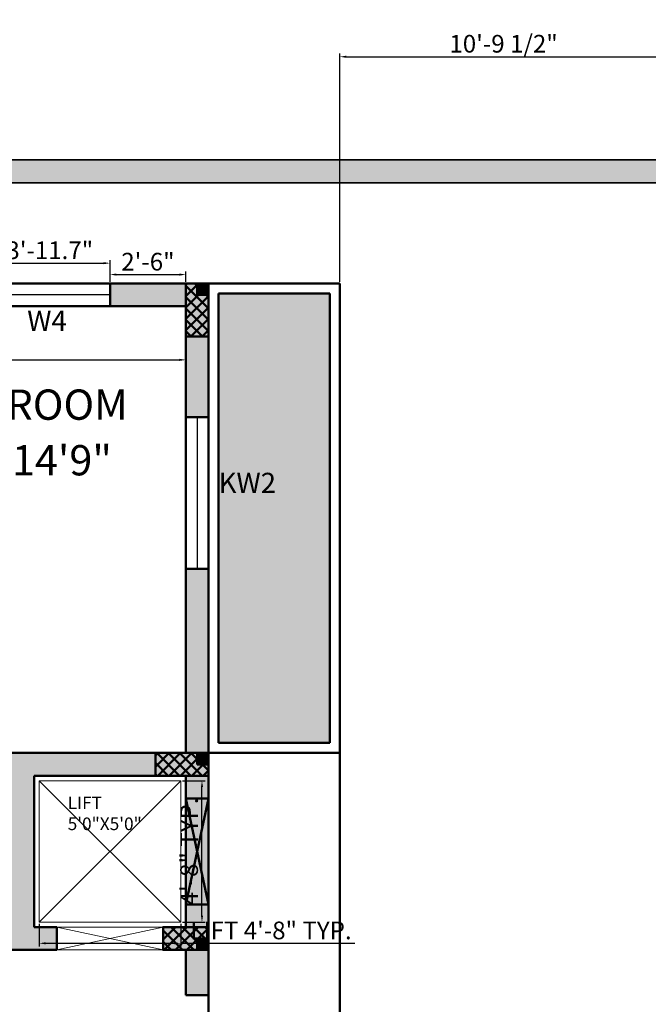
# Model space of a CAD drawing. Units: inches. Extents: x 1749 to 3550, y 1117 to 2383.
# Tile 8 of 15: x 2038 to 2287, y 1993 to 2383. Entities that reach past the tile are written whole.
import ezdxf

# ---------------------------------------------------------------- set-up
doc = ezdxf.new("R2010")
doc.units = ezdxf.units.IN
for name, color, linetype, lineweight in [('A-ANNO-DIMS', 2, 'Continuous', 18), ('A-ANNO-TEXT', 3, 'Continuous', 18), ('A-AREA-IDEN', 7, 'Continuous', 18), ('A-COLS', 10, 'Continuous', 50), ('A-EQPM', 8, 'Continuous', 18), ('A-GLAZ', 4, 'Continuous', 25), ('A-WALL', 7, 'Continuous', 50), ('A-WALL-PATT', 8, 'Continuous', 13), ('C-PROP', 8, 'Continuous', 35)]:
    doc.layers.add(name, color=color, linetype=linetype, lineweight=lineweight)
doc.styles.get("Standard").update_dxf_attribs({"font": 'arial.ttf'})
doc.dimstyles.new('ISO-25', dxfattribs={"dimtxt": 7, "dimasz": 2.5, "dimexe": 1.25, "dimexo": 0.625, "dimtad": 1, "dimdec": 1, "dimlunit": 3, "dimtxsty": 'Standard', "dimcen": 2.5, "dimadec": 0, "dimazin": 0, "dimtfac": 1, "dimtdec": 1, "dimtmove": 0, "dimatfit": 3, "dimfxl": 1, "dimarcsym": 0})

# ---------------------------------------------------------------- blocks, each defined once
blk = doc.blocks.new('*D5')
at = {"layer": 'A-ANNO-DIMS', "color": 0, "lineweight": -2, "transparency": 16777216}
for p, q in [((1868.6, 2249.04), (1868.6, 2249.66)), ((1871.1, 2248.41), (2101.6, 2248.41)), ((2104.1, 2249.04), (2104.1, 2249.66))]:
    blk.add_line(p, q, dxfattribs=at)
at = {"layer": 'A-ANNO-DIMS', "color": 0, "transparency": 16777216}
for points in [[(1871.1, 2248.83), (1871.1, 2247.99), (1868.6, 2248.41)], [(2101.6, 2248.83), (2101.6, 2247.99), (2104.1, 2248.41)]]:
    blk.add_solid(points, dxfattribs=at)
at = {"layer": 'Defpoints', "color": 0, "transparency": 16777216}
for p in [(1868.6, 2248.41), (2104.1, 2248.41), (2104.1, 2248.41)]:
    blk.add_point(p, dxfattribs=at)
at = {"layer": 'A-ANNO-DIMS', "color": 0, "transparency": 16777216, "insert": (1986.35, 2252.61), "char_height": 7, "attachment_point": 5}
blk.add_mtext('19\'-7.5"', dxfattribs=at)
blk = doc.blocks.new('*D76')
at = {"layer": 'A-ANNO-DIMS', "color": 0, "lineweight": -2, "ltscale": 0.5, "transparency": 16777216}
for p, q in [((2026.42, 2279.29), (2026.42, 2287.96)), ((2028.92, 2286.71), (2071.6, 2286.71)), ((2074.1, 2279.29), (2074.1, 2287.96))]:
    blk.add_line(p, q, dxfattribs=at)
at = {"layer": 'A-ANNO-DIMS', "color": 0, "ltscale": 0.5, "transparency": 16777216}
for points in [[(2028.92, 2287.12), (2028.92, 2286.29), (2026.42, 2286.71)], [(2071.6, 2287.12), (2071.6, 2286.29), (2074.1, 2286.71)]]:
    blk.add_solid(points, dxfattribs=at)
at = {"layer": 'Defpoints', "color": 0, "ltscale": 0.5, "transparency": 16777216}
for p in [(2074.1, 2286.71), (2026.42, 2278.66), (2074.1, 2278.66)]:
    blk.add_point(p, dxfattribs=at)
at = {"layer": 'A-ANNO-DIMS', "color": 0, "ltscale": 0.5, "transparency": 16777216, "insert": (2050.26, 2290.91), "char_height": 7, "attachment_point": 5}
blk.add_mtext('3\'-11.7"', dxfattribs=at)
blk = doc.blocks.new('*D77')
at = {"layer": 'A-ANNO-DIMS', "color": 0, "lineweight": -2, "ltscale": 0.5, "transparency": 16777216}
for p, q in [((2074.1, 2279.29), (2074.1, 2283.44)), ((2076.6, 2282.19), (2101.6, 2282.19)), ((2104.1, 2279.29), (2104.1, 2283.44))]:
    blk.add_line(p, q, dxfattribs=at)
at = {"layer": 'A-ANNO-DIMS', "color": 0, "ltscale": 0.5, "transparency": 16777216}
for points in [[(2076.6, 2282.61), (2076.6, 2281.77), (2074.1, 2282.19)], [(2101.6, 2282.61), (2101.6, 2281.77), (2104.1, 2282.19)]]:
    blk.add_solid(points, dxfattribs=at)
at = {"layer": 'Defpoints', "color": 0, "ltscale": 0.5, "transparency": 16777216}
for p in [(2104.1, 2282.19), (2074.1, 2278.66), (2104.1, 2278.66)]:
    blk.add_point(p, dxfattribs=at)
at = {"layer": 'A-ANNO-DIMS', "color": 0, "ltscale": 0.5, "transparency": 16777216, "insert": (2089.1, 2286.39), "char_height": 7, "attachment_point": 5}
blk.add_mtext('2\'-6"', dxfattribs=at)
blk = doc.blocks.new('LIFT-A')
at = {"ltscale": 0.2}
for p, q in [((0, 56), (56, 56)), ((0, 56), (0, 0)), ((56, 56), (0, 0)), ((0, 56), (56, 0)), ((56, 56), (56, 0)), ((0, 0), (56, 0))]:
    blk.add_line(p, q, dxfattribs=at)
blk = doc.blocks.new('*D153')
at = {"layer": 'A-ANNO-DIMS', "color": 0, "lineweight": -2, "ltscale": 0.5, "transparency": 16777216}
for p, q in [((2046.1, 2025.04), (2046.1, 2016.01)), ((2102.1, 2025.04), (2102.1, 2016.01)), ((2048.6, 2017.26), (2099.6, 2017.26)), ((2102.1, 2017.26), (2171.03, 2017.26))]:
    blk.add_line(p, q, dxfattribs=at)
at = {"layer": 'A-ANNO-DIMS', "color": 0, "ltscale": 0.5, "transparency": 16777216}
for points in [[(2048.6, 2017.68), (2048.6, 2016.84), (2046.1, 2017.26)], [(2099.6, 2017.68), (2099.6, 2016.84), (2102.1, 2017.26)]]:
    blk.add_solid(points, dxfattribs=at)
at = {"layer": 'Defpoints', "color": 0, "ltscale": 0.5, "transparency": 16777216}
for p in [(2046.1, 2025.66), (2102.1, 2025.66), (2102.1, 2017.26)]:
    blk.add_point(p, dxfattribs=at)
at = {"layer": 'A-ANNO-DIMS', "color": 0, "ltscale": 0.5, "transparency": 16777216, "insert": (2137.82, 2021.46), "char_height": 7, "attachment_point": 5}
blk.add_mtext('LIFT 4\'-8" TYP.', dxfattribs=at)
blk = doc.blocks.new('*D154')
at = {"layer": 'A-ANNO-DIMS', "color": 0, "lineweight": -2, "ltscale": 0.5, "transparency": 16777216}
for p, q in [((2102.73, 2081.66), (2111.75, 2081.66)), ((2110.5, 2028.16), (2110.5, 2079.16)), ((2102.73, 2025.66), (2111.75, 2025.66))]:
    blk.add_line(p, q, dxfattribs=at)
at = {"layer": 'A-ANNO-DIMS', "color": 0, "ltscale": 0.5, "transparency": 16777216}
for points in [[(2110.09, 2079.16), (2110.92, 2079.16), (2110.5, 2081.66)], [(2110.09, 2028.16), (2110.92, 2028.16), (2110.5, 2025.66)]]:
    blk.add_solid(points, dxfattribs=at)
at = {"layer": 'Defpoints', "color": 0, "ltscale": 0.5, "transparency": 16777216}
for p in [(2102.1, 2081.66), (2110.5, 2081.66), (2102.1, 2025.66)]:
    blk.add_point(p, dxfattribs=at)
at = {"layer": 'A-ANNO-DIMS', "color": 0, "ltscale": 0.5, "transparency": 16777216, "insert": (2106.31, 2053.66), "char_height": 7, "attachment_point": 5, "rotation": 90}
blk.add_mtext('4\'-8" TYP.', dxfattribs=at)
blk = doc.blocks.new('*D164')
at = {"layer": 'A-ANNO-DIMS', "color": 0, "lineweight": -2, "ltscale": 0.5, "transparency": 16777216}
for p, q in [((2165.1, 2279.29), (2165.1, 2369.73)), ((2167.6, 2368.48), (2292.1, 2368.48)), ((2294.6, 2278.29), (2294.6, 2369.73))]:
    blk.add_line(p, q, dxfattribs=at)
at = {"layer": 'A-ANNO-DIMS', "color": 0, "ltscale": 0.5, "transparency": 16777216}
for points in [[(2167.6, 2368.9), (2167.6, 2368.06), (2165.1, 2368.48)], [(2292.1, 2368.9), (2292.1, 2368.06), (2294.6, 2368.48)]]:
    blk.add_solid(points, dxfattribs=at)
at = {"layer": 'Defpoints', "color": 0, "ltscale": 0.5, "transparency": 16777216}
for p in [(2294.6, 2368.48), (2165.1, 2278.66), (2294.6, 2277.66)]:
    blk.add_point(p, dxfattribs=at)
at = {"layer": 'A-ANNO-DIMS', "color": 0, "ltscale": 0.5, "transparency": 16777216, "insert": (2229.85, 2372.73), "char_height": 7, "attachment_point": 5}
blk.add_mtext('10\'-9 1/2"', dxfattribs=at)

msp = doc.modelspace()

# ---------------------------------------------------------------- hatches: boundary and pattern name
at = {"layer": 'A-COLS'}
h = msp.add_hatch(dxfattribs=at)
h.set_pattern_fill('ANSI37', color=256, angle=-90)
h.set_pattern_definition([(315, (332.5445, 4525.2253), (2.245064, 2.245064), []), (45, (332.5445, 4525.2253), (-2.245064, 2.245064), [])])
h.paths.add_polyline_path([(2113.1, 2278.66), (2104.1, 2278.66), (2104.1, 2257.66), (2113.1, 2257.66)])
h = msp.add_hatch(color=256, dxfattribs=at)
h.dxf.hatch_style = 1
h.paths.add_polyline_path([(2108.6, 2274.16), (2113.1, 2274.16), (2113.1, 2278.66), (2108.6, 2278.66)])
h = msp.add_hatch(dxfattribs=at)
h.set_pattern_fill('ANSI37', color=256)
h.set_pattern_definition([(45, (-154.4595, 312.1017), (-2.245064, 2.245064), []), (135, (-154.4595, 312.1017), (-2.245064, -2.245064), [])])
h.paths.add_polyline_path([(2092.1, 2092.66), (2092.1, 2083.66), (2113.1, 2083.66), (2113.1, 2092.66)])
h = msp.add_hatch(color=256, dxfattribs=at)
h.dxf.hatch_style = 1
h.paths.add_polyline_path([(2108.6, 2088.16), (2113.1, 2088.16), (2113.1, 2092.66), (2108.6, 2092.66)])
h = msp.add_hatch(dxfattribs=at)
h.set_pattern_fill('ANSI37', color=256)
h.paths.add_polyline_path([(2113.1, 2023.66), (2095.1, 2023.66), (2095.1, 2014.66), (2108.6, 2014.66), (2108.6, 2019.16), (2113.1, 2019.16)])
h = msp.add_hatch(color=256, dxfattribs=at)
h.dxf.hatch_style = 1
h.paths.add_polyline_path([(2108.6, 2014.66), (2113.1, 2014.66), (2113.1, 2019.16), (2108.6, 2019.16)])
at = {"layer": 'A-WALL-PATT', "ltscale": 0.5}
h = msp.add_hatch(color=256, dxfattribs=at)
h.dxf.hatch_style = 1
h.paths.add_polyline_path([(2612.84, 2327.58), (1804.37, 2327.58), (1804.37, 1803), (2612.84, 1803), (2612.84, 2093.66), (2603.84, 2093.66), (2603.84, 1812), (1813.37, 1812), (1813.37, 2318.58), (2603.84, 2318.58), (2603.84, 2268.45), (2612.84, 2268.45)])
at = {"layer": 'A-WALL-PATT'}
h = msp.add_hatch(color=256, dxfattribs=at)
h.dxf.hatch_style = 1
h.paths.add_polyline_path([(2113.1, 2278.66), (2074.1, 2278.66), (2074.1, 2269.66), (2104.1, 2269.66), (2104.1, 2225.66), (2113.1, 2225.66)])
h = msp.add_hatch(color=256, dxfattribs=at)
h.dxf.hatch_style = 1
h.paths.add_polyline_path([(2161.1, 2274.66), (2117.1, 2274.66), (2117.1, 2096.66), (2161.1, 2096.66)])
h.paths.add_polyline_path([(2161.1, 1944.66), (2117.1, 1944.66), (2117.1, 1853.66), (2161.1, 1853.66)])
h = msp.add_hatch(color=256, dxfattribs=at)
h.dxf.hatch_style = 1
h.paths.add_polyline_path([(2113.1, 2092.66), (2104.1, 2092.66), (1927.1, 2092.66), (1927.1, 2181.16), (1868.6, 2181.16), (1868.6, 2187.16), (1859.6, 2187.16), (1859.6, 2170.66), (1868.6, 2170.66), (1868.6, 2176.66), (1922.6, 2176.66), (1922.6, 2092.66), (1868.6, 2092.66), (1868.6, 2110.66), (1859.6, 2110.66), (1859.6, 2083.66), (1922.6, 2083.66), (1922.6, 2065.66), (1927.1, 2065.66), (1927.1, 2083.66), (2035.1, 2083.66), (2035.1, 2023.66), (2029.1, 2023.66), (2029.1, 2014.66), (2053.1, 2014.66), (2053.1, 2023.66), (2044.1, 2023.66), (2044.1, 2083.66), (2104.1, 2083.66), (2104.1, 2023.66), (2095.1, 2023.66), (2095.1, 2014.66), (2104.1, 2014.66), (2104.1, 1996.66), (2113.1, 1996.66)])
h = msp.add_hatch(color=256, dxfattribs=at)
h.dxf.hatch_style = 1
h.paths.add_polyline_path([(2113.1, 2165.66), (2104.1, 2165.66), (2104.1, 2092.66), (2113.1, 2092.66)])

# ---------------------------------------------------------------- linework, layer by layer
at = {"layer": 'A-COLS'}
for p, q in [((2108.6, 2278.66), (2108.6, 2274.16)), ((2113.1, 2278.66), (2108.6, 2278.66)), ((2113.1, 2274.16), (2113.1, 2278.66)), ((2108.6, 2274.16), (2113.1, 2274.16)), ((2108.6, 2092.66), (2108.6, 2088.16)), ((2113.1, 2092.66), (2108.6, 2092.66)), ((2113.1, 2088.16), (2113.1, 2092.66)), ((2108.6, 2088.16), (2113.1, 2088.16)), ((2113.1, 2074.66), (2104.1, 2074.66)), ((2104.1, 2074.66), (2104.1, 2032.66)), ((2113.1, 2074.66), (2104.1, 2032.66)), ((2104.1, 2074.66), (2113.1, 2032.66)), ((2113.1, 2074.66), (2113.1, 2032.66)), ((2113.1, 2032.66), (2104.1, 2032.66)), ((2108.6, 2019.16), (2108.6, 2014.66)), ((2113.1, 2019.16), (2108.6, 2019.16)), ((2113.1, 2014.66), (2113.1, 2019.16)), ((2108.6, 2014.66), (2113.1, 2014.66))]:
    msp.add_line(p, q, dxfattribs=at)
for points in [[(2113.1, 2278.66), (2113.1, 2257.66), (2104.1, 2257.66), (2104.1, 2278.66)], [(2092.1, 2092.66), (2113.1, 2092.66), (2113.1, 2083.66), (2092.1, 2083.66)], [(2113.1, 2014.66), (2095.1, 2014.66), (2095.1, 2023.66), (2113.1, 2023.66)]]:
    msp.add_lwpolyline(points, close=True, dxfattribs=at)
at = {"layer": 'A-EQPM', "ltscale": 0.2}
for p, q in [((2053.1, 2014.66), (2053.1, 2023.66)), ((2053.1, 2023.66), (2095.1, 2014.66)), ((2095.1, 2023.66), (2053.1, 2014.66)), ((2095.1, 2023.66), (2053.1, 2023.66)), ((2095.1, 2023.66), (2095.1, 2014.66)), ((2095.1, 2014.66), (2095.1, 2023.66)), ((2095.1, 2014.66), (2053.1, 2014.66))]:
    msp.add_line(p, q, dxfattribs=at)
at = {"layer": 'A-GLAZ'}
for p, q in [((2074.1, 2274.16), (2026.1, 2274.16)), ((2108.6, 2225.66), (2108.6, 2165.66))]:
    msp.add_line(p, q, dxfattribs=at)
at = {"layer": 'A-WALL'}
for p, q in [((1859.6, 2278.66), (2113.1, 2278.66)), ((2074.1, 2269.66), (2074.1, 2278.66)), ((2113.1, 2278.66), (2113.1, 1948.66)), ((2113.1, 2278.66), (2165.1, 2278.66)), ((2165.1, 2278.66), (2165.1, 1849.66)), ((2117.1, 2274.66), (2117.1, 2096.66)), ((2117.1, 2274.66), (2161.1, 2274.66)), ((2161.1, 2274.66), (2161.1, 2096.66)), ((1868.6, 2269.66), (2104.1, 2269.66)), ((2104.1, 2269.66), (2104.1, 2092.66)), ((2104.1, 2225.66), (2113.1, 2225.66)), ((2104.1, 2165.66), (2113.1, 2165.66)), ((2117.1, 2096.66), (2161.1, 2096.66)), ((1927.1, 2092.66), (2104.1, 2092.66)), ((2113.1, 2092.66), (2165.1, 2092.66)), ((2044.1, 2083.66), (2104.1, 2083.66)), ((2044.1, 2083.66), (2044.1, 2023.66)), ((2104.1, 2083.66), (2104.1, 2023.66)), ((2044.1, 2023.66), (2053.1, 2023.66)), ((2044.1, 2023.66), (2053.1, 2023.66)), ((2053.1, 2023.66), (2053.1, 2014.66)), ((2095.1, 2023.66), (2104.1, 2023.66)), ((2095.1, 2023.66), (2095.1, 2014.66)), ((2095.1, 2023.66), (2104.1, 2023.66)), ((2029.1, 2014.66), (2053.1, 2014.66)), ((2095.1, 2014.66), (2104.1, 2014.66)), ((2104.1, 2014.66), (2104.1, 1996.66)), ((2104.1, 1996.66), (2113.1, 1996.66))]:
    msp.add_line(p, q, dxfattribs=at)
at = {"layer": 'C-PROP', "ltscale": 0.5}
for p, q in [((1804.37, 2327.58), (2612.84, 2327.58)), ((1813.37, 2318.58), (2603.84, 2318.58))]:
    msp.add_line(p, q, dxfattribs=at)

# ---------------------------------------------------------------- block references
at = {"layer": 'A-EQPM'}
msp.add_blockref('LIFT-A', (2046.1, 2025.66), dxfattribs=at)

# ---------------------------------------------------------------- texts
at = {"layer": 'A-ANNO-TEXT', "ltscale": 0.5}
for s, p in [('W4', (2041.34, 2259.9)), ('KW2', (2117.1, 2195.66))]:
    msp.add_text(s, height=8, dxfattribs=at).set_placement(p)
at = {"layer": 'A-AREA-IDEN', "ltscale": 0.5}
msp.add_text('SERVANT ROOM', height=12, rotation=0.0333, dxfattribs=at).set_placement((1958.68, 2224.61))
for s, height, p in [('19\'8"X14\'9"', 12, (1986.35, 2202.64)), ('LIFT', 5, (2057.36, 2070.41)), ('5\'0"X5\'0"', 5, (2057.36, 2062.11))]:
    msp.add_text(s, height=height, dxfattribs=at).set_placement(p)

# ---------------------------------------------------------------- dimensions: what is measured, and where the dimension line sits
at = {"layer": 'A-ANNO-DIMS', "ltscale": 0.5}
for base, p1, p2, override, picture, middle in [((2294.6, 2368.48), (2165.1, 2278.66), (2294.6, 2277.66), {"dimdec": 1, "dimlfac": 1, "dimrnd": 0, "dimzin": 1, "dimdsep": 46, "dimlunit": 4, "dimfrac": 2}, '*D164', (2229.85, 2372.73)), ((2074.1, 2286.71), (2026.42, 2278.66), (2074.1, 2278.66), {"dimclrd": 0, "dimclre": 0, "dimclrt": 0}, '*D76', (2050.26, 2290.91)), ((2104.1, 2282.19), (2074.1, 2278.66), (2104.1, 2278.66), {"dimclrd": 0, "dimclre": 0, "dimclrt": 0}, '*D77', (2089.1, 2286.39))]:
    dim = msp.add_linear_dim(base=base, p1=p1, p2=p2, dimstyle='ISO-25', override=override, dxfattribs=at)
    dim.commit()
    dim.dimension.update_dxf_attribs({"geometry": picture, "text_midpoint": middle})
at = {"layer": 'A-ANNO-DIMS'}
dim = msp.add_linear_dim(base=(2104.1, 2248.41), p1=(1868.6, 2248.41), p2=(2104.1, 2248.41), dimstyle='ISO-25', override={"dimclrd": 0, "dimclre": 0, "dimclrt": 0}, dxfattribs=at)
dim.commit()
dim.dimension.update_dxf_attribs({"geometry": '*D5', "text_midpoint": (1986.35, 2252.61)})
at = {"layer": 'A-ANNO-DIMS', "ltscale": 0.5}
dim = msp.add_linear_dim(base=(2110.5, 2081.66), p1=(2102.1, 2025.66), p2=(2102.1, 2081.66), angle=90, text='<> TYP.', dimstyle='ISO-25', override={"dimdec": 1, "dimrnd": 0, "dimzin": 1, "dimlunit": 4, "dimfrac": 2}, dxfattribs=at)
dim.commit()
dim.dimension.update_dxf_attribs({"geometry": '*D154', "text_midpoint": (2106.31, 2053.66)})
dim = msp.add_linear_dim(base=(2102.1, 2017.26), p1=(2046.1, 2025.66), p2=(2102.1, 2025.66), text='LIFT <> TYP.', dimstyle='ISO-25', override={"dimdec": 1, "dimrnd": 0, "dimzin": 1, "dimlunit": 4, "dimfrac": 2}, dxfattribs=at)
dim.commit()
dim.dimension.update_dxf_attribs({"geometry": '*D153', "text_midpoint": (2137.82, 2021.46)})

doc.saveas('drawing.dxf')
